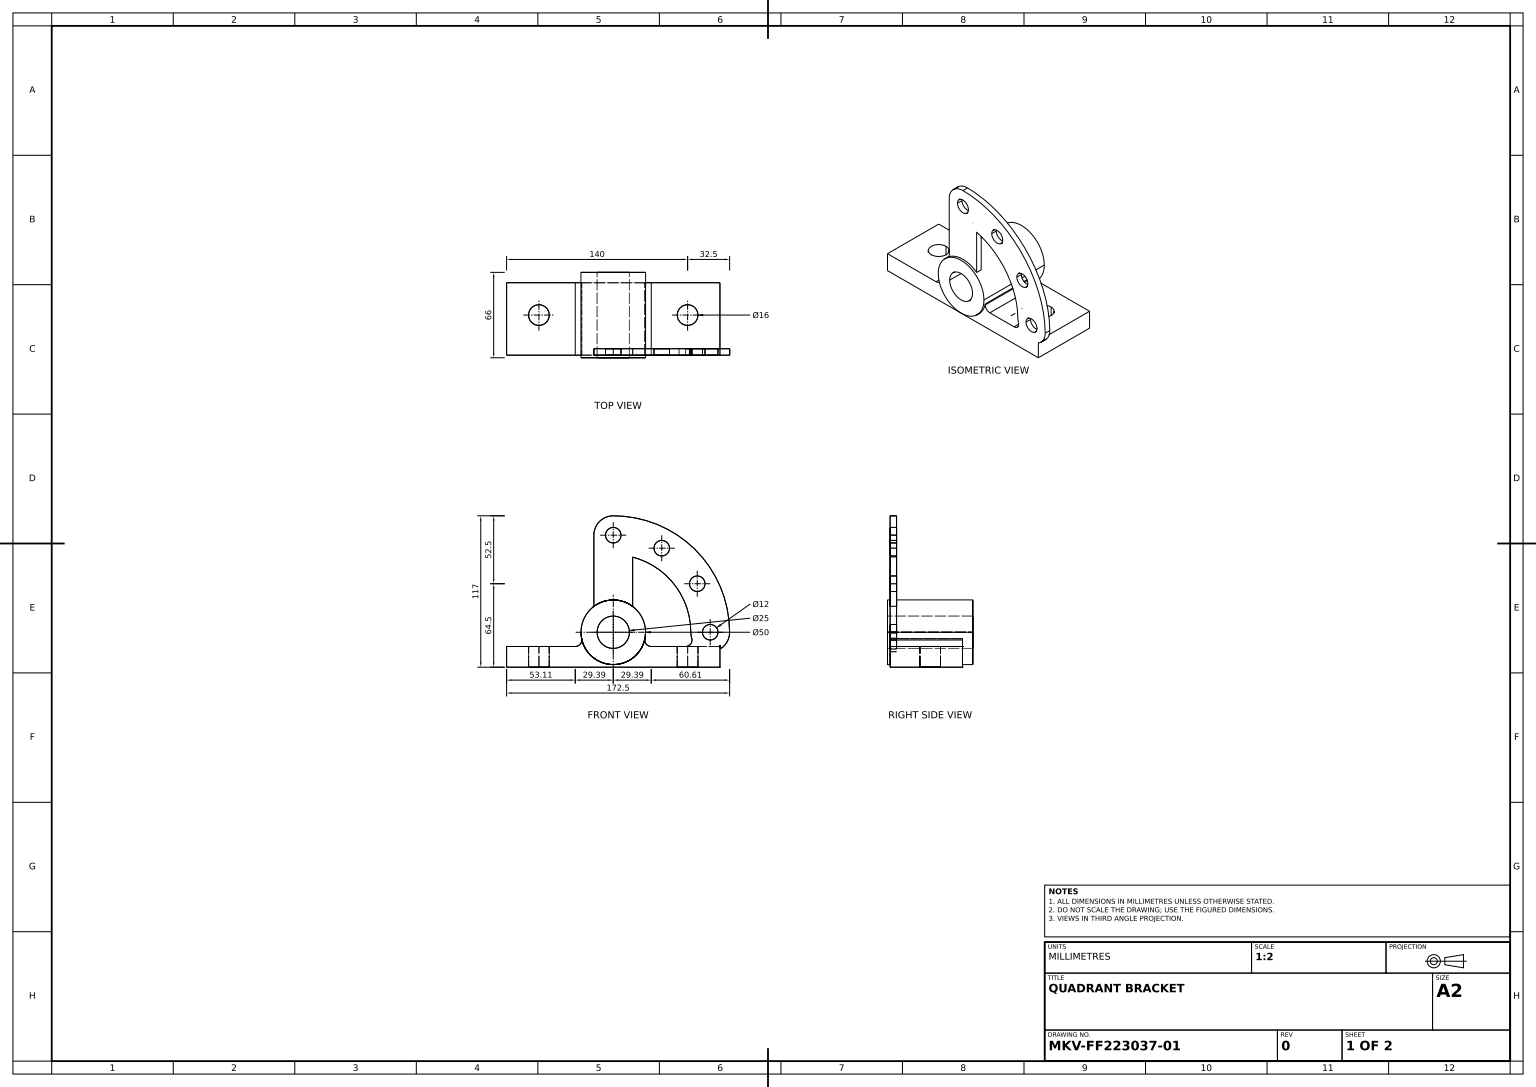
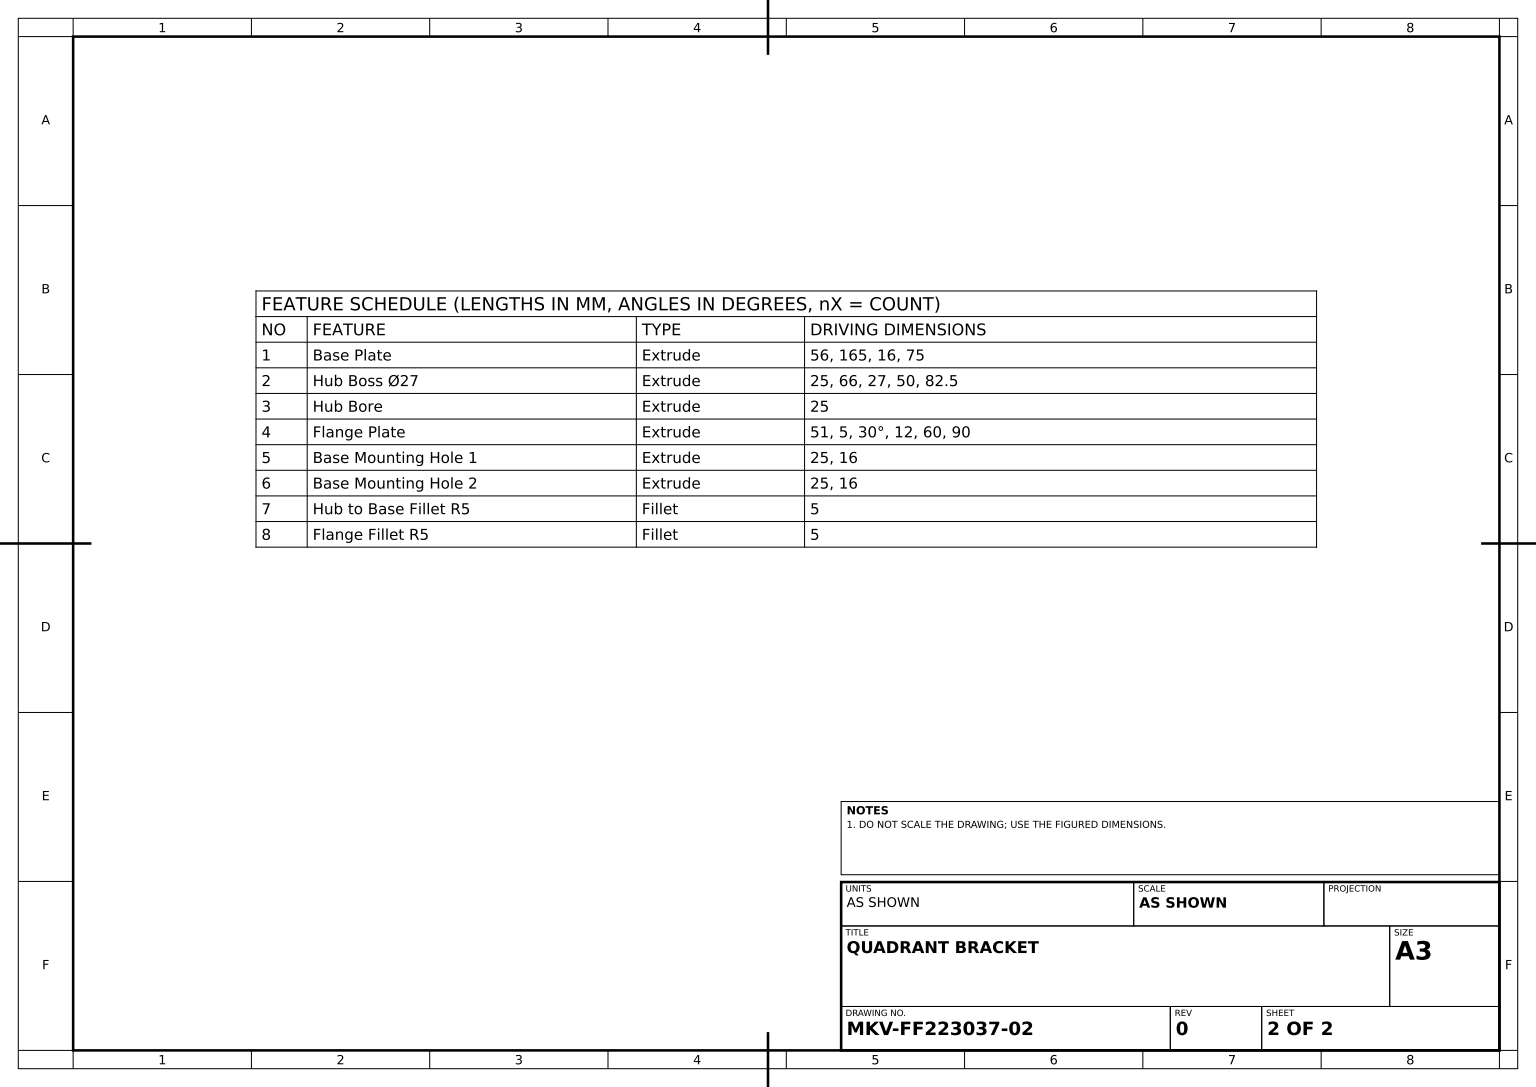
SolidWorks part; units mm, degrees
material "Plain Carbon Steel"
ref_plane "Front Plane" through (0, 0, 0) normal (0, 0, 1) x (1, 0, 0)
ref_plane "Top Plane" through (0, 0, 0) normal (0, 1, 0) x (1, 0, 0)
ref_plane "Right Plane" through (0, 0, 0) normal (1, 0, 0) x (0, 0, -1)
sketch "Base Plate Profile" plane through (0, 0, 0) normal (0, 0, 1) x (1, 0, 0)
  line L0 (0, 0) -> (75, 0)
  line L1 (75, 0) -> (165, 0)
  line L2 (165, 0) -> (165, 16)
  line L3 (165, 16) -> (0, 16)
  line L4 (0, 16) -> (0, 0)
  dimension "D1" = 165
  dimension "D2" = 16
  dimension "D3" = 75
extrude "Base Plate" add sketch "Base Plate Profile" along normal blind 56
ref_plane "Plane3" through (0, 0, 28) normal (0, 0, 1) x (1, 0, 0)
ref_plane "Plane4" through (0, 0, 51) normal (0, 0, 1) x (1, 0, 0)
ref_plane "Plane5" through (0, 0, 25) normal (0, 0, 1) x (1, 0, 0)
sketch "Hub Boss Profile" plane through (0, 0, 25) normal (0, 0, 1) x (1, 0, 0)
  line L0 (0, 0) -> (165, 0) construction
  circle A0 centre (82.5, 27) radius 25
  circle A1 centre (82.5, 27) radius 12.5
  dimension "D1" = 27
  dimension "D2" = 50
  dimension "D3" = 25
  dimension "D4" = 82.5
extrude "Hub Boss Ø27" add sketch "Hub Boss Profile" along normal mid plane 66
sketch "Hub Bore Profile" plane through (0, 0, 58) normal (0, 0, 1) x (1, 0, 0)
  circle A0 centre (82.5, 27) radius 12.5
  dimension "D1" = 25
extrude "Hub Bore" cut sketch "Hub Bore Profile" against normal through all
ref_plane "Plane6" through (0, 0, 51) normal (0, 0, 1) x (1, 0, 0)
sketch "Flange Plate Profile" plane through (0, 0, 51) normal (0, 0, 1) x (1, 0, 0)
  line L0 (82.5, 27) -> (82.5, 117) construction
  line L1 (82.5, 27) -> (157.5, 27) construction
  line L2 (67.5, 102) -> (67.5, 47)
  line L3 (97.5, 85.0948) -> (97.5, 47)
  line L4 (82.5, 27) -> (147.4519, 64.5) construction
  line L5 (97.5, 102) -> (97.5, 47) construction
  line L7 (82.5, 27) -> (120, 91.9519) construction
  arc A0 (142.5, 27) -> (82.5, 87) centre (82.5, 27) ccw
  arc A1 (172.5, 27) -> (82.5, 117) centre (82.5, 27) ccw
  arc A2 (157.5, 27) -> (82.5, 102) centre (82.5, 27) ccw construction
  arc A3 (82.5, 117) -> (82.5, 87) centre (82.5, 102) ccw
  arc A4 (142.5, 27) -> (172.5, 27) centre (157.5, 27) ccw
  circle A5 centre (82.5, 27) radius 25 construction
  arc A6 (97.5, 47) -> (67.5, 47) centre (82.5, 27) ccw
  circle A7 centre (82.5, 102) radius 6
  circle A8 centre (157.5, 27) radius 6
  circle A9 centre (147.4519, 64.5) radius 6
  circle A10 centre (120, 91.9519) radius 6
  dimension "D1" = 30
  dimension "D3" = 12
  dimension "D4" = 60
  dimension "D5" = 90
  dimension "D2" = 30
extrude "Flange Plate" add sketch "Flange Plate Profile" along normal blind 5 contours A6 L3 A0 A3 L2 | A0 A4 A1 A3 A10 A9 A8 A7
sketch "Base Mounting Hole 1 Profile" plane through (0, 16, 0) normal (0, 1, 0) x (1, 0, 0)
  line L0 (60.0501, 0) -> (0, 0) construction
  line L1 (0, -56) -> (0, 0) construction
  circle A0 centre (25, -25) radius 8
  dimension "D1" = 25
  dimension "D3" = 16
  dimension "D2" = 25
extrude "Base Mounting Hole 1" cut sketch "Base Mounting Hole 1 Profile" against normal through all
sketch "Base Mounting Hole 2 Profile" plane through (0, 16, 0) normal (0, 1, 0) x (1, 0, 0)
  line L0 (165, 0) -> (104.9499, 0) construction
  line L1 (165, -51) -> (165, 0) construction
  circle A0 centre (140, -25) radius 8
  dimension "D1" = 25
  dimension "D3" = 16
  dimension "D2" = 25
extrude "Base Mounting Hole 2" cut sketch "Base Mounting Hole 2 Profile" against normal through all
fillet "Hub to Base Fillet R5" radius 5 1 edges at (60.0501, 16, 28)
fillet "Flange Fillet R5" radius 5 2 edges at (147.302, 16, 53.5) (104.9499, 16, 28)
